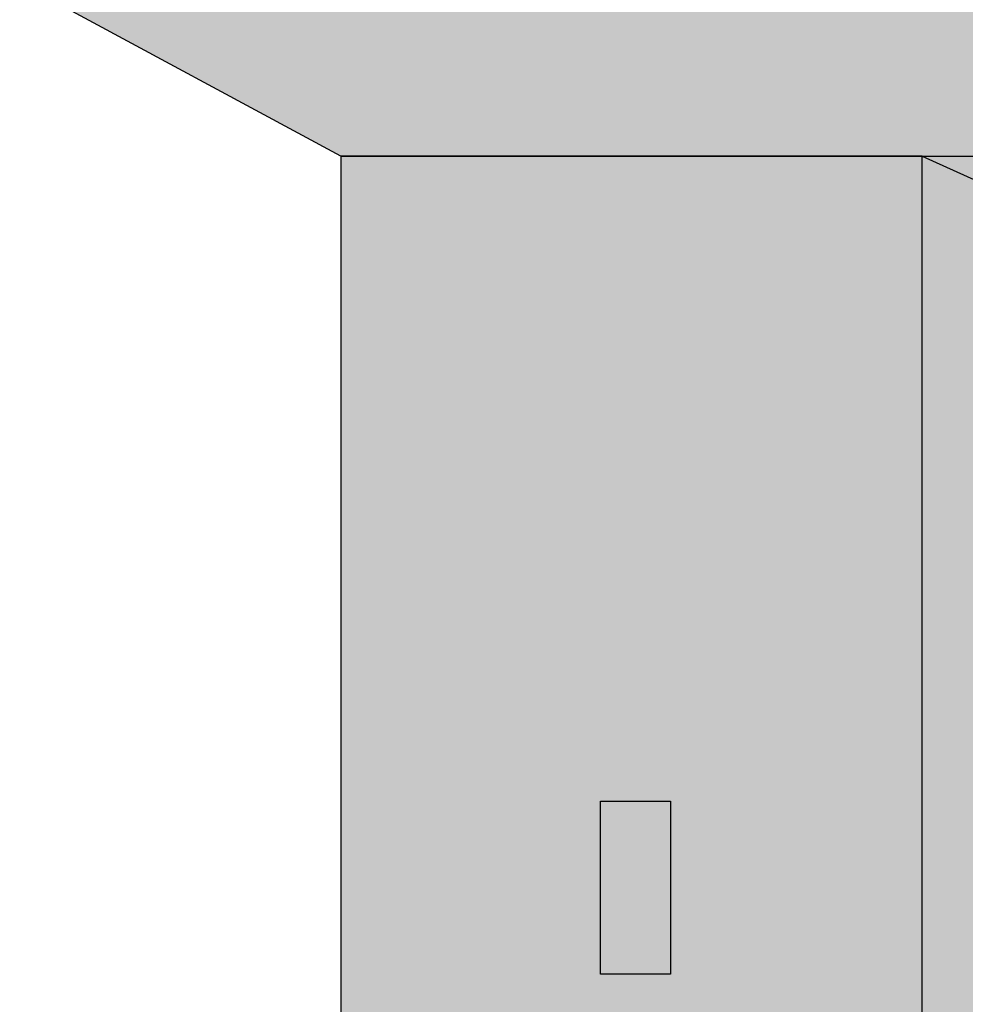
# Model space of a CAD drawing. Units: feet. Extents: x 2368 to 3224, y 836 to 1229.
# Tile 4 of 9: x 2368 to 2447, y 903 to 985. Entities that reach past the tile are written whole.
import ezdxf

# ---------------------------------------------------------------- set-up
doc = ezdxf.new("R2010")
doc.units = ezdxf.units.FT
doc.layers.add('A-ELEV', color=7, linetype='Continuous', lineweight=25)
doc.layers.add('A-ELEV-PATT', color=8, linetype='Continuous', lineweight=13)

msp = doc.modelspace()

# ---------------------------------------------------------------- hatches: boundary and pattern name
at = {"layer": 'A-ELEV-PATT'}
h = msp.add_hatch(color=256, dxfattribs=at)
h.dxf.hatch_style = 1
h.paths.add_polyline_path([(2584.596, 1202.153), (2582.106, 1202.153), (2582.106, 1108.749), (2584.596, 1108.749)])
h.paths.add_polyline_path([(2656.206, 1202.153), (2653.716, 1202.153), (2653.716, 1108.749), (2656.206, 1108.749)])
h.paths.add_polyline_path([(2693.729, 1040.781), (2656.206, 1040.781), (2656.206, 1099.51), (2653.716, 1099.51), (2653.716, 1040.781), (2584.596, 1040.781), (2584.596, 1099.51), (2582.106, 1099.51), (2582.106, 1040.781), (2544.984, 1040.781), (2544.984, 1040.065), (2582.106, 1040.065), (2582.106, 1037.139), (2544.984, 1037.139), (2544.984, 1036.769), (2582.106, 1036.769), (2582.106, 1033.485), (2544.984, 1033.485), (2544.984, 1033.114), (2582.106, 1033.114), (2582.106, 1029.831), (2544.984, 1029.831), (2544.984, 1029.46), (2582.106, 1029.46), (2582.106, 1026.176), (2544.984, 1026.176), (2544.984, 1025.806), (2582.106, 1025.806), (2582.106, 1022.522), (2544.984, 1022.522), (2544.984, 1022.151), (2582.106, 1022.151), (2582.106, 1018.868), (2544.984, 1018.868), (2544.984, 1018.497), (2582.106, 1018.497), (2582.106, 1015.213), (2544.984, 1015.213), (2544.984, 1014.843), (2582.106, 1014.843), (2582.106, 1011.559), (2544.984, 1011.559), (2544.984, 1011.188), (2582.106, 1011.188), (2582.106, 1007.905), (2544.984, 1007.905), (2544.984, 1007.534), (2582.106, 1007.534), (2582.106, 1006.105), (2584.596, 1006.105), (2584.596, 1007.534), (2619.488, 1007.534), (2619.488, 1006.105), (2620.425, 1006.105), (2620.425, 1007.534), (2653.716, 1007.534), (2653.716, 1006.105), (2656.206, 1006.105), (2656.206, 1007.534), (2693.729, 1007.534), (2693.729, 1007.905), (2656.206, 1007.905), (2656.206, 1011.188), (2693.729, 1011.188), (2693.729, 1011.559), (2656.206, 1011.559), (2656.206, 1014.843), (2693.729, 1014.843), (2693.729, 1015.213), (2656.206, 1015.213), (2656.206, 1018.497), (2693.729, 1018.497), (2693.729, 1018.868), (2656.206, 1018.868), (2656.206, 1022.151), (2693.729, 1022.151), (2693.729, 1022.522), (2656.206, 1022.522), (2656.206, 1025.806), (2693.729, 1025.806), (2693.729, 1026.176), (2656.206, 1026.176), (2656.206, 1029.46), (2693.729, 1029.46), (2693.729, 1029.831), (2656.206, 1029.831), (2656.206, 1033.114), (2693.729, 1033.114), (2693.729, 1033.485), (2656.206, 1033.485), (2656.206, 1036.769), (2693.729, 1036.769), (2693.729, 1037.139), (2656.206, 1037.139), (2656.206, 1040.065), (2693.729, 1040.065)])
h.paths.add_polyline_path([(2584.596, 1040.065), (2619.488, 1040.065), (2619.488, 1037.139), (2584.596, 1037.139)], flags=16)
h.paths.add_polyline_path([(2584.596, 1036.769), (2619.488, 1036.769), (2619.488, 1033.485), (2584.596, 1033.485)], flags=16)
h.paths.add_polyline_path([(2584.596, 1033.114), (2619.488, 1033.114), (2619.488, 1029.831), (2584.596, 1029.831)], flags=16)
h.paths.add_polyline_path([(2584.596, 1029.46), (2619.488, 1029.46), (2619.488, 1026.176), (2584.596, 1026.176)], flags=16)
h.paths.add_polyline_path([(2584.596, 1025.806), (2619.488, 1025.806), (2619.488, 1022.522), (2584.596, 1022.522)], flags=16)
h.paths.add_polyline_path([(2584.596, 1022.151), (2619.488, 1022.151), (2619.488, 1018.868), (2584.596, 1018.868)], flags=16)
h.paths.add_polyline_path([(2584.596, 1018.497), (2619.488, 1018.497), (2619.488, 1015.213), (2584.596, 1015.213)], flags=16)
h.paths.add_polyline_path([(2584.596, 1014.843), (2619.488, 1014.843), (2619.488, 1011.559), (2584.596, 1011.559)], flags=16)
h.paths.add_polyline_path([(2584.596, 1011.188), (2619.488, 1011.188), (2619.488, 1007.905), (2584.596, 1007.905)], flags=16)
h.paths.add_polyline_path([(2620.425, 1040.065), (2653.716, 1040.065), (2653.716, 1037.139), (2620.425, 1037.139)], flags=16)
h.paths.add_polyline_path([(2620.425, 1036.769), (2653.716, 1036.769), (2653.716, 1033.485), (2620.425, 1033.485)], flags=16)
h.paths.add_polyline_path([(2620.425, 1033.114), (2653.716, 1033.114), (2653.716, 1029.831), (2620.425, 1029.831)], flags=16)
h.paths.add_polyline_path([(2620.425, 1029.46), (2653.716, 1029.46), (2653.716, 1026.176), (2620.425, 1026.176)], flags=16)
h.paths.add_polyline_path([(2620.425, 1025.806), (2653.716, 1025.806), (2653.716, 1022.522), (2620.425, 1022.522)], flags=16)
h.paths.add_polyline_path([(2620.425, 1022.151), (2653.716, 1022.151), (2653.716, 1018.868), (2620.425, 1018.868)], flags=16)
h.paths.add_polyline_path([(2620.425, 1018.497), (2653.716, 1018.497), (2653.716, 1015.213), (2620.425, 1015.213)], flags=16)
h.paths.add_polyline_path([(2620.425, 1014.843), (2653.716, 1014.843), (2653.716, 1011.559), (2620.425, 1011.559)], flags=16)
h.paths.add_polyline_path([(2620.425, 1011.188), (2653.716, 1011.188), (2653.716, 1007.905), (2620.425, 1007.905)], flags=16)
h.paths.add_polyline_path([(2536.7, 926.195), (2529.874, 926.195), (2529.874, 904.71), (2536.7, 904.71)])
h.paths.add_polyline_path([(2422.205, 920.108), (2416.403, 920.108), (2416.403, 905.784), (2422.205, 905.784)])
h = msp.add_hatch(color=256, dxfattribs=at)
h.dxf.hatch_style = 1
h.paths.add_polyline_path([(2443.042, 973.51), (2394.909, 973.51), (2394.909, 853.51), (2443.042, 853.51)])
h.paths.add_polyline_path([(2422.205, 920.108), (2422.205, 905.784), (2416.403, 905.784), (2416.403, 920.108)], flags=16)
h.paths.add_polyline_path([(2449.299, 970.694), (2443.042, 973.51), (2443.042, 853.51), (2449.299, 853.51)])
h.paths.add_polyline_path([(2510.022, 987.861), (2368.302, 987.861), (2394.909, 973.51), (2443.042, 973.51), (2510.022, 973.51)])
h.paths.add_polyline_path([(2510.022, 973.51), (2443.042, 973.51), (2449.299, 970.694), (2510.022, 970.694)])

# ---------------------------------------------------------------- linework, layer by layer
at = {"layer": 'A-ELEV'}
for p, q in [((2394.909, 973.51), (2368.302, 987.861)), ((2394.909, 973.51), (2368.302, 987.861)), ((2394.909, 973.51), (2510.022, 973.51)), ((2394.909, 973.51), (2510.022, 973.51)), ((2443.042, 973.51), (2449.299, 970.694)), ((2443.042, 973.51), (2449.299, 970.694))]:
    msp.add_line(p, q, dxfattribs=at)
for points in [[(2394.909, 853.51), (2443.042, 853.51), (2443.042, 973.51), (2394.909, 973.51)], [(2394.909, 853.51), (2443.042, 853.51), (2443.042, 973.51), (2394.909, 973.51)], [(2416.403, 920.108), (2422.205, 920.108), (2422.205, 905.784), (2416.403, 905.784)], [(2416.403, 920.108), (2422.205, 920.108), (2422.205, 905.784), (2416.403, 905.784)]]:
    msp.add_lwpolyline(points, close=True, dxfattribs=at)

doc.saveas('drawing.dxf')
